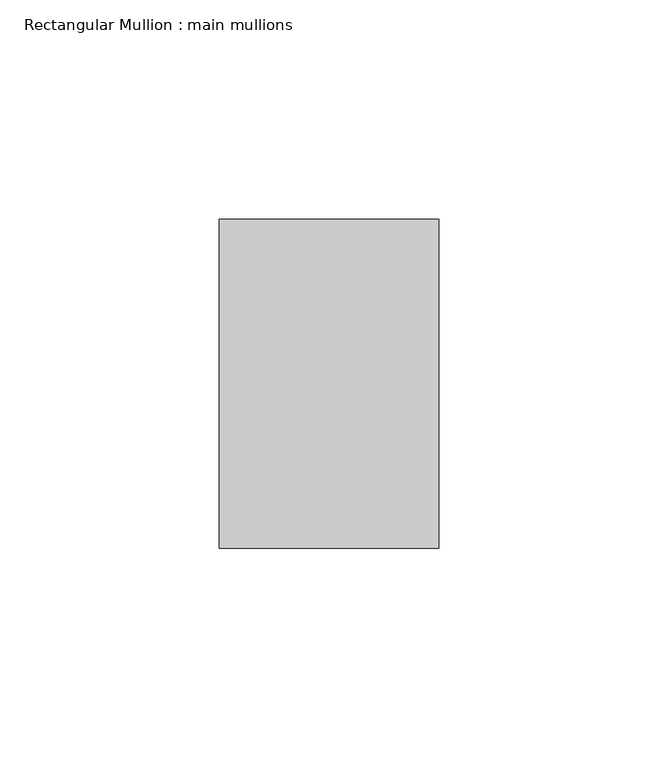
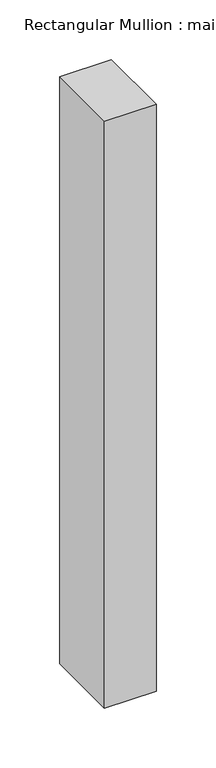
"""IFC4 building model written with IfcOpenShell, lengths in millimetres: member geometry, Rectangular Mullion : main mullions."""

from ifc_helpers import new_model, si_unit, frame, origin, place, context, project, spatial, polyline, outline, extrude, source, transform, mapped, element, save


def rectangular_mullion_main_mullions_fa6a4a93(model_context):
    return source(origin(), model_context, "Body", "SweptSolid", [
        extrude(outline(polyline([(0.0, 37.5), (0.0, -37.5), (-50.0, -37.5), (-50.0, 37.5), (0.0, 37.5)])), frame((0.0, 0.0, -600.0), z_axis=(0.0, 0.0, 1.0), x_axis=(1.0, 0.0, 0.0)), (0.0, 0.0, 1.0), 600.0),
    ])


if __name__ == "__main__":
    model = new_model("IFC4")
    model_context = context("Model", 3, world=origin())
    ifc_project = project(units=[si_unit("LENGTHUNIT", "METRE", prefix="MILLI")], contexts=[model_context])
    site = spatial("IfcSite", under=ifc_project)
    building = spatial("IfcBuilding", under=site)
    placement = place(None, origin())
    rectangular_mullion_main_mullions_shape = rectangular_mullion_main_mullions_fa6a4a93(model_context)
    element("IfcMember", 1, ObjectType="Rectangular Mullion : main mullions", at=placement, inside=building, context=model_context, shape_type="MappedRepresentation", body=[
        mapped(rectangular_mullion_main_mullions_shape, transform((0.0, 0.0, 0.0), x_axis=(1.0, 0.0, 0.0), y_axis=(0.0, 1.0, 0.0), z_axis=(0.0, 0.0, 1.0))),
    ])
    save(model, "model.ifc")

# Revit data of these elements
# Type "Rectangular Mullion : main mullions"
#   built-in parameter 1007304 = 0.246063 (stored number, unit not read)
#   built-in parameter 1007301 = 0.082021 (stored number, unit not read)
#   built-in parameter 1007300 = 0.082021 (stored number, unit not read)
# Element 1 (IfcMember, "Rectangular Mullion : main mullions")
#   Materials on its faces: "Aluminum"
# Materials
#   "Aluminum": class "Metal", colour RGB 136 136 136, transparency 0, Description = "Aluminum 6061", Cost = 0
